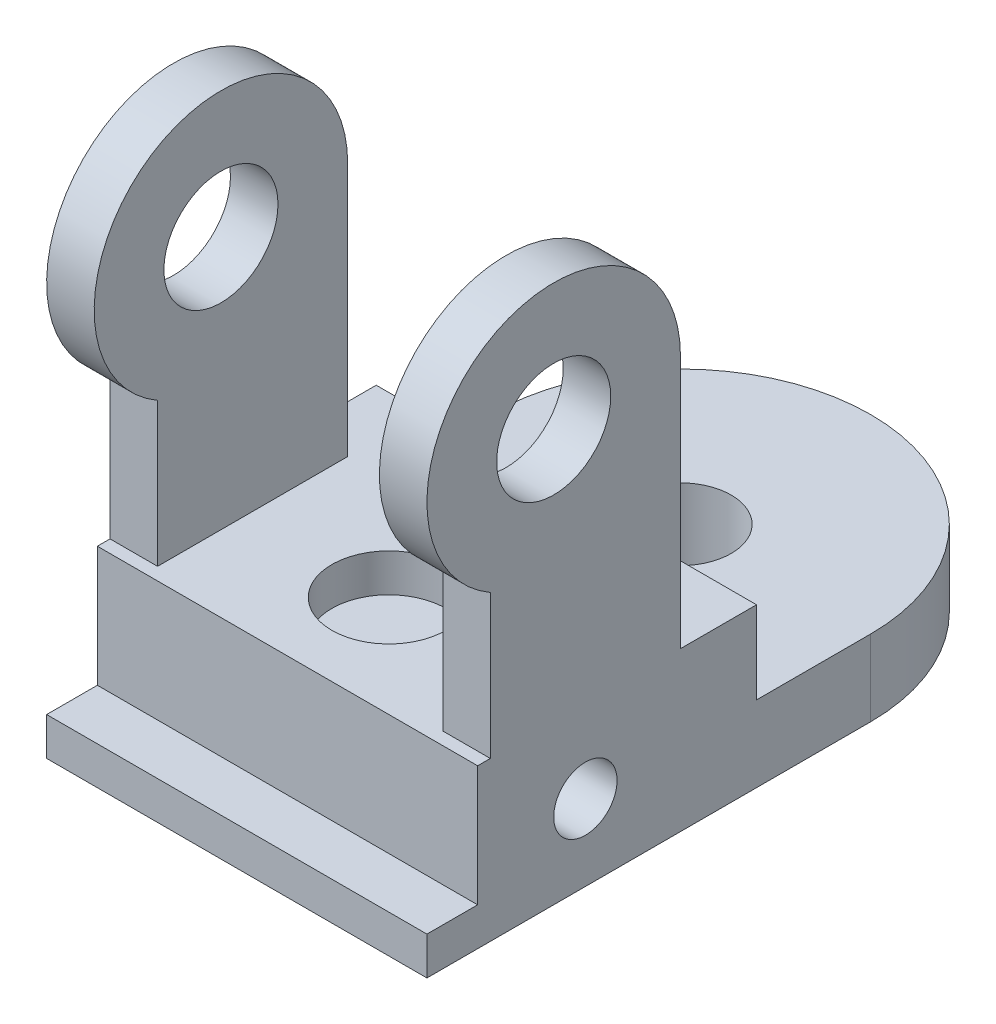
ISO-10303-21;
HEADER;
FILE_DESCRIPTION(('STEP AP214'),'2;1');
FILE_NAME('part.step','',(''),(''),'','','');
FILE_SCHEMA(('AUTOMOTIVE_DESIGN { 1 0 10303 214 1 1 1 1 }'));
ENDSEC;
DATA;
#1=APPLICATION_CONTEXT('core data for automotive mechanical design processes');
#2=APPLICATION_PROTOCOL_DEFINITION('international standard','automotive_design',2000,#1);
#3=PRODUCT_CONTEXT('',#1,'mechanical');
#4=PRODUCT('Part','Part','',(#3));
#5=PRODUCT_RELATED_PRODUCT_CATEGORY('part','',(#4));
#6=PRODUCT_DEFINITION_FORMATION('','',#4);
#7=PRODUCT_DEFINITION_CONTEXT('part definition',#1,'design');
#8=PRODUCT_DEFINITION('design','',#6,#7);
#9=PRODUCT_DEFINITION_SHAPE('','',#8);
#10=(LENGTH_UNIT() NAMED_UNIT(*) SI_UNIT(.MILLI.,.METRE.));
#11=(NAMED_UNIT(*) PLANE_ANGLE_UNIT() SI_UNIT($,.RADIAN.));
#12=(NAMED_UNIT(*) SI_UNIT($,.STERADIAN.) SOLID_ANGLE_UNIT());
#13=UNCERTAINTY_MEASURE_WITH_UNIT(LENGTH_MEASURE(1.E-05),#10,'distance_accuracy_value','');
#14=(GEOMETRIC_REPRESENTATION_CONTEXT(3) GLOBAL_UNCERTAINTY_ASSIGNED_CONTEXT((#13)) GLOBAL_UNIT_ASSIGNED_CONTEXT((#10,
#11,#12)) REPRESENTATION_CONTEXT('',''));
#15=CARTESIAN_POINT('',(0.,0.,0.));
#16=DIRECTION('',(0.,0.,1.));
#17=DIRECTION('',(1.,0.,0.));
#18=AXIS2_PLACEMENT_3D('',#15,#16,#17);
#19=CARTESIAN_POINT('',(-30.,0.,18.));
#20=DIRECTION('',(0.,0.,-1.));
#21=DIRECTION('',(-1.,0.,0.));
#22=AXIS2_PLACEMENT_3D('',#19,#20,#21);
#23=PLANE('',#22);
#24=CARTESIAN_POINT('',(0.,25.,18.));
#25=DIRECTION('',(0.,0.,-1.));
#26=DIRECTION('',(-1.,0.,0.));
#27=AXIS2_PLACEMENT_3D('',#24,#25,#26);
#28=CIRCLE('',#27,13.);
#29=CARTESIAN_POINT('',(13.,25.,18.));
#30=VERTEX_POINT('',#29);
#31=CARTESIAN_POINT('',(0.,12.,18.));
#32=VERTEX_POINT('',#31);
#33=EDGE_CURVE('E47',#30,#32,#28,.T.);
#34=ORIENTED_EDGE('',*,*,#33,.F.);
#35=DIRECTION('',(1.,0.,0.));
#36=VECTOR('',#35,1.);
#37=CARTESIAN_POINT('',(-30.,25.,18.));
#38=LINE('',#37,#36);
#39=CARTESIAN_POINT('',(30.,25.,18.));
#40=VERTEX_POINT('',#39);
#41=EDGE_CURVE('E183',#30,#40,#38,.T.);
#42=ORIENTED_EDGE('',*,*,#41,.T.);
#43=DIRECTION('',(0.,1.,0.));
#44=VECTOR('',#43,1.);
#45=CARTESIAN_POINT('',(30.,0.,18.));
#46=LINE('',#45,#44);
#47=CARTESIAN_POINT('',(30.,12.,18.));
#48=VERTEX_POINT('',#47);
#49=EDGE_CURVE('E252',#48,#40,#46,.T.);
#50=ORIENTED_EDGE('',*,*,#49,.F.);
#51=DIRECTION('',(1.,0.,0.));
#52=VECTOR('',#51,1.);
#53=CARTESIAN_POINT('',(-30.,12.,18.));
#54=LINE('',#53,#52);
#55=EDGE_CURVE('E261',#32,#48,#54,.T.);
#56=ORIENTED_EDGE('',*,*,#55,.F.);
#57=EDGE_LOOP('',(#34,#42,#50,#56));
#58=FACE_BOUND('',#57,.T.);
#59=ADVANCED_FACE('F41',(#58),#23,.T.);
#60=CARTESIAN_POINT('',(-30.,25.,0.));
#61=DIRECTION('',(0.,1.,0.));
#62=DIRECTION('',(0.,0.,1.));
#63=AXIS2_PLACEMENT_3D('',#60,#61,#62);
#64=PLANE('',#63);
#65=CARTESIAN_POINT('',(0.,25.,46.));
#66=DIRECTION('',(0.,1.,0.));
#67=DIRECTION('',(0.,0.,1.));
#68=AXIS2_PLACEMENT_3D('',#65,#66,#67);
#69=CIRCLE('',#68,9.);
#70=CARTESIAN_POINT('',(0.,25.,55.));
#71=VERTEX_POINT('',#70);
#72=EDGE_CURVE('E451',#71,#71,#69,.T.);
#73=ORIENTED_EDGE('',*,*,#72,.F.);
#74=EDGE_LOOP('',(#73));
#75=FACE_BOUND('',#74,.T.);
#76=DIRECTION('',(0.,0.,-1.));
#77=VECTOR('',#76,1.);
#78=CARTESIAN_POINT('',(13.,25.,30.));
#79=LINE('',#78,#77);
#80=CARTESIAN_POINT('',(13.,25.,30.));
#81=VERTEX_POINT('',#80);
#82=EDGE_CURVE('E174',#81,#30,#79,.T.);
#83=ORIENTED_EDGE('',*,*,#82,.F.);
#84=DIRECTION('',(-1.,0.,0.));
#85=VECTOR('',#84,1.);
#86=CARTESIAN_POINT('',(-30.,25.,30.));
#87=LINE('',#86,#85);
#88=CARTESIAN_POINT('',(-13.,25.,30.));
#89=VERTEX_POINT('',#88);
#90=EDGE_CURVE('E11',#81,#89,#87,.T.);
#91=ORIENTED_EDGE('',*,*,#90,.T.);
#92=DIRECTION('',(0.,0.,-1.));
#93=VECTOR('',#92,1.);
#94=CARTESIAN_POINT('',(-13.,25.,30.));
#95=LINE('',#94,#93);
#96=CARTESIAN_POINT('',(-13.,25.,18.));
#97=VERTEX_POINT('',#96);
#98=EDGE_CURVE('E166',#97,#89,#95,.F.);
#99=ORIENTED_EDGE('',*,*,#98,.F.);
#100=CARTESIAN_POINT('',(-30.,25.,18.));
#101=VERTEX_POINT('',#100);
#102=EDGE_CURVE('E273',#101,#97,#38,.T.);
#103=ORIENTED_EDGE('',*,*,#102,.F.);
#104=DIRECTION('',(0.,0.,1.));
#105=VECTOR('',#104,1.);
#106=CARTESIAN_POINT('',(-30.,25.,0.));
#107=LINE('',#106,#105);
#108=CARTESIAN_POINT('',(-30.,25.,30.));
#109=VERTEX_POINT('',#108);
#110=EDGE_CURVE('E262',#101,#109,#107,.T.);
#111=ORIENTED_EDGE('',*,*,#110,.T.);
#112=DIRECTION('',(-1.,0.,0.));
#113=VECTOR('',#112,1.);
#114=CARTESIAN_POINT('',(-22.5,25.,30.));
#115=LINE('',#114,#113);
#116=CARTESIAN_POINT('',(-22.5,25.,30.));
#117=VERTEX_POINT('',#116);
#118=EDGE_CURVE('E202',#117,#109,#115,.T.);
#119=ORIENTED_EDGE('',*,*,#118,.F.);
#120=DIRECTION('',(0.,0.,1.));
#121=VECTOR('',#120,1.);
#122=CARTESIAN_POINT('',(-22.5,25.,0.));
#123=LINE('',#122,#121);
#124=CARTESIAN_POINT('',(-22.5,25.,60.));
#125=VERTEX_POINT('',#124);
#126=EDGE_CURVE('E65',#117,#125,#123,.T.);
#127=ORIENTED_EDGE('',*,*,#126,.T.);
#128=DIRECTION('',(-1.,0.,0.));
#129=VECTOR('',#128,1.);
#130=CARTESIAN_POINT('',(-22.5,25.,60.));
#131=LINE('',#130,#129);
#132=CARTESIAN_POINT('',(-30.,25.,60.));
#133=VERTEX_POINT('',#132);
#134=EDGE_CURVE('E217',#125,#133,#131,.T.);
#135=ORIENTED_EDGE('',*,*,#134,.T.);
#136=CARTESIAN_POINT('',(-30.,25.,62.));
#137=VERTEX_POINT('',#136);
#138=EDGE_CURVE('E263',#133,#137,#107,.T.);
#139=ORIENTED_EDGE('',*,*,#138,.T.);
#140=DIRECTION('',(1.,0.,0.));
#141=VECTOR('',#140,1.);
#142=CARTESIAN_POINT('',(-30.,25.,62.));
#143=LINE('',#142,#141);
#144=CARTESIAN_POINT('',(30.,25.,62.));
#145=VERTEX_POINT('',#144);
#146=EDGE_CURVE('E272',#137,#145,#143,.T.);
#147=ORIENTED_EDGE('',*,*,#146,.T.);
#148=DIRECTION('',(0.,0.,1.));
#149=VECTOR('',#148,1.);
#150=CARTESIAN_POINT('',(30.,25.,0.));
#151=LINE('',#150,#149);
#152=CARTESIAN_POINT('',(30.,25.,60.));
#153=VERTEX_POINT('',#152);
#154=EDGE_CURVE('E267',#153,#145,#151,.T.);
#155=ORIENTED_EDGE('',*,*,#154,.F.);
#156=DIRECTION('',(1.,0.,0.));
#157=VECTOR('',#156,1.);
#158=CARTESIAN_POINT('',(22.5,25.,60.));
#159=LINE('',#158,#157);
#160=CARTESIAN_POINT('',(22.5,25.,60.));
#161=VERTEX_POINT('',#160);
#162=EDGE_CURVE('E255',#161,#153,#159,.T.);
#163=ORIENTED_EDGE('',*,*,#162,.F.);
#164=DIRECTION('',(0.,0.,1.));
#165=VECTOR('',#164,1.);
#166=CARTESIAN_POINT('',(22.5,25.,0.));
#167=LINE('',#166,#165);
#168=CARTESIAN_POINT('',(22.5,25.,30.));
#169=VERTEX_POINT('',#168);
#170=EDGE_CURVE('E234',#169,#161,#167,.T.);
#171=ORIENTED_EDGE('',*,*,#170,.F.);
#172=DIRECTION('',(1.,0.,0.));
#173=VECTOR('',#172,1.);
#174=CARTESIAN_POINT('',(22.5,25.,30.));
#175=LINE('',#174,#173);
#176=CARTESIAN_POINT('',(30.,25.,30.));
#177=VERTEX_POINT('',#176);
#178=EDGE_CURVE('E247',#169,#177,#175,.T.);
#179=ORIENTED_EDGE('',*,*,#178,.T.);
#180=EDGE_CURVE('E264',#40,#177,#151,.T.);
#181=ORIENTED_EDGE('',*,*,#180,.F.);
#182=ORIENTED_EDGE('',*,*,#41,.F.);
#183=EDGE_LOOP('',(#83,#91,#99,#103,#111,#119,#127,#135,#139,#147,#155,#163,#171,#179,#181,#182));
#184=FACE_BOUND('',#183,.T.);
#185=ADVANCED_FACE('F181',(#75,#184),#64,.T.);
#186=CARTESIAN_POINT('',(0.,12.,0.));
#187=DIRECTION('',(0.,1.,0.));
#188=DIRECTION('',(0.,0.,1.));
#189=AXIS2_PLACEMENT_3D('',#186,#187,#188);
#190=PLANE('',#189);
#191=CARTESIAN_POINT('',(0.,12.,0.));
#192=DIRECTION('',(0.,1.,0.));
#193=DIRECTION('',(0.,0.,1.));
#194=AXIS2_PLACEMENT_3D('',#191,#192,#193);
#195=CIRCLE('',#194,8.);
#196=CARTESIAN_POINT('',(0.,12.,8.));
#197=VERTEX_POINT('',#196);
#198=EDGE_CURVE('E292',#197,#197,#195,.T.);
#199=ORIENTED_EDGE('',*,*,#198,.F.);
#200=EDGE_LOOP('',(#199));
#201=FACE_BOUND('',#200,.T.);
#202=DIRECTION('',(0.,0.,1.));
#203=VECTOR('',#202,1.);
#204=CARTESIAN_POINT('',(-30.,12.,70.));
#205=LINE('',#204,#203);
#206=CARTESIAN_POINT('',(-30.,12.,0.));
#207=VERTEX_POINT('',#206);
#208=CARTESIAN_POINT('',(-30.,12.,18.));
#209=VERTEX_POINT('',#208);
#210=EDGE_CURVE('E302',#207,#209,#205,.T.);
#211=ORIENTED_EDGE('',*,*,#210,.T.);
#212=EDGE_CURVE('E276',#209,#32,#54,.T.);
#213=ORIENTED_EDGE('',*,*,#212,.T.);
#214=ORIENTED_EDGE('',*,*,#55,.T.);
#215=DIRECTION('',(0.,0.,-1.));
#216=VECTOR('',#215,1.);
#217=CARTESIAN_POINT('',(30.,12.,0.));
#218=LINE('',#217,#216);
#219=CARTESIAN_POINT('',(30.,12.,0.));
#220=VERTEX_POINT('',#219);
#221=EDGE_CURVE('E308',#48,#220,#218,.T.);
#222=ORIENTED_EDGE('',*,*,#221,.T.);
#223=CARTESIAN_POINT('',(0.,12.,0.));
#224=DIRECTION('',(0.,1.,0.));
#225=DIRECTION('',(0.,0.,1.));
#226=AXIS2_PLACEMENT_3D('',#223,#224,#225);
#227=CIRCLE('',#226,30.);
#228=EDGE_CURVE('E301',#220,#207,#227,.T.);
#229=ORIENTED_EDGE('',*,*,#228,.T.);
#230=EDGE_LOOP('',(#211,#213,#214,#222,#229));
#231=FACE_BOUND('',#230,.T.);
#232=ADVANCED_FACE('F378',(#201,#231),#190,.T.);
#233=CARTESIAN_POINT('',(30.,12.,70.));
#234=DIRECTION('',(0.,0.,-1.));
#235=DIRECTION('',(-1.,0.,0.));
#236=AXIS2_PLACEMENT_3D('',#233,#234,#235);
#237=PLANE('',#236);
#238=DIRECTION('',(1.,0.,0.));
#239=VECTOR('',#238,1.);
#240=CARTESIAN_POINT('',(-30.,6.,70.));
#241=LINE('',#240,#239);
#242=CARTESIAN_POINT('',(-30.,6.,70.));
#243=VERTEX_POINT('',#242);
#244=CARTESIAN_POINT('',(30.,6.,70.));
#245=VERTEX_POINT('',#244);
#246=EDGE_CURVE('E283',#243,#245,#241,.T.);
#247=ORIENTED_EDGE('',*,*,#246,.F.);
#248=DIRECTION('',(0.,-1.,0.));
#249=VECTOR('',#248,1.);
#250=CARTESIAN_POINT('',(-30.,12.,70.));
#251=LINE('',#250,#249);
#252=CARTESIAN_POINT('',(-30.,0.,70.));
#253=VERTEX_POINT('',#252);
#254=EDGE_CURVE('E323',#243,#253,#251,.T.);
#255=ORIENTED_EDGE('',*,*,#254,.T.);
#256=DIRECTION('',(1.,0.,0.));
#257=VECTOR('',#256,1.);
#258=CARTESIAN_POINT('',(30.,0.,70.));
#259=LINE('',#258,#257);
#260=CARTESIAN_POINT('',(30.,0.,70.));
#261=VERTEX_POINT('',#260);
#262=EDGE_CURVE('E317',#253,#261,#259,.T.);
#263=ORIENTED_EDGE('',*,*,#262,.T.);
#264=DIRECTION('',(0.,-1.,0.));
#265=VECTOR('',#264,1.);
#266=CARTESIAN_POINT('',(30.,12.,70.));
#267=LINE('',#266,#265);
#268=EDGE_CURVE('E321',#245,#261,#267,.T.);
#269=ORIENTED_EDGE('',*,*,#268,.F.);
#270=EDGE_LOOP('',(#247,#255,#263,#269));
#271=FACE_BOUND('',#270,.T.);
#272=ADVANCED_FACE('F348',(#271),#237,.F.);
#273=CARTESIAN_POINT('',(0.,12.,0.));
#274=DIRECTION('',(0.,-1.,0.));
#275=DIRECTION('',(0.,0.,-1.));
#276=AXIS2_PLACEMENT_3D('',#273,#274,#275);
#277=CYLINDRICAL_SURFACE('',#276,30.);
#278=CARTESIAN_POINT('',(0.,0.,0.));
#279=DIRECTION('',(0.,1.,0.));
#280=DIRECTION('',(0.,0.,1.));
#281=AXIS2_PLACEMENT_3D('',#278,#279,#280);
#282=CIRCLE('',#281,30.);
#283=CARTESIAN_POINT('',(30.,0.,0.));
#284=VERTEX_POINT('',#283);
#285=CARTESIAN_POINT('',(-30.,0.,0.));
#286=VERTEX_POINT('',#285);
#287=EDGE_CURVE('E296',#284,#286,#282,.T.);
#288=ORIENTED_EDGE('',*,*,#287,.T.);
#289=DIRECTION('',(0.,-1.,0.));
#290=VECTOR('',#289,1.);
#291=CARTESIAN_POINT('',(-30.,12.,0.));
#292=LINE('',#291,#290);
#293=EDGE_CURVE('E328',#207,#286,#292,.T.);
#294=ORIENTED_EDGE('',*,*,#293,.F.);
#295=ORIENTED_EDGE('',*,*,#228,.F.);
#296=DIRECTION('',(0.,-1.,0.));
#297=VECTOR('',#296,1.);
#298=CARTESIAN_POINT('',(30.,12.,0.));
#299=LINE('',#298,#297);
#300=EDGE_CURVE('E309',#220,#284,#299,.T.);
#301=ORIENTED_EDGE('',*,*,#300,.T.);
#302=EDGE_LOOP('',(#288,#294,#295,#301));
#303=FACE_BOUND('',#302,.T.);
#304=ADVANCED_FACE('F43',(#303),#277,.T.);
#305=CARTESIAN_POINT('',(-30.,12.,70.));
#306=DIRECTION('',(1.,0.,0.));
#307=DIRECTION('',(0.,0.,-1.));
#308=AXIS2_PLACEMENT_3D('',#305,#306,#307);
#309=PLANE('',#308);
#310=CARTESIAN_POINT('',(-30.,12.,45.));
#311=DIRECTION('',(-1.,0.,0.));
#312=DIRECTION('',(0.,0.,1.));
#313=AXIS2_PLACEMENT_3D('',#310,#311,#312);
#314=CIRCLE('',#313,5.);
#315=CARTESIAN_POINT('',(-30.,12.,50.));
#316=VERTEX_POINT('',#315);
#317=EDGE_CURVE('E450',#316,#316,#314,.T.);
#318=ORIENTED_EDGE('',*,*,#317,.F.);
#319=EDGE_LOOP('',(#318));
#320=FACE_BOUND('',#319,.T.);
#321=DIRECTION('',(0.,0.,1.));
#322=VECTOR('',#321,1.);
#323=CARTESIAN_POINT('',(-30.,6.,62.));
#324=LINE('',#323,#322);
#325=CARTESIAN_POINT('',(-30.,6.,62.));
#326=VERTEX_POINT('',#325);
#327=EDGE_CURVE('E274',#326,#243,#324,.T.);
#328=ORIENTED_EDGE('',*,*,#327,.F.);
#329=DIRECTION('',(0.,1.,0.));
#330=VECTOR('',#329,1.);
#331=CARTESIAN_POINT('',(-30.,6.,62.));
#332=LINE('',#331,#330);
#333=EDGE_CURVE('E290',#326,#137,#332,.T.);
#334=ORIENTED_EDGE('',*,*,#333,.T.);
#335=ORIENTED_EDGE('',*,*,#138,.F.);
#336=DIRECTION('',(0.,1.,0.));
#337=VECTOR('',#336,1.);
#338=CARTESIAN_POINT('',(-30.,0.,60.));
#339=LINE('',#338,#337);
#340=CARTESIAN_POINT('',(-30.,47.6794919243112,60.));
#341=VERTEX_POINT('',#340);
#342=EDGE_CURVE('E210',#133,#341,#339,.T.);
#343=ORIENTED_EDGE('',*,*,#342,.T.);
#344=CARTESIAN_POINT('',(-30.,65.,50.));
#345=DIRECTION('',(1.,0.,0.));
#346=DIRECTION('',(0.,0.,-1.));
#347=AXIS2_PLACEMENT_3D('',#344,#345,#346);
#348=CIRCLE('',#347,20.);
#349=CARTESIAN_POINT('',(-30.,65.,30.));
#350=VERTEX_POINT('',#349);
#351=EDGE_CURVE('E192',#350,#341,#348,.T.);
#352=ORIENTED_EDGE('',*,*,#351,.F.);
#353=DIRECTION('',(0.,1.,0.));
#354=VECTOR('',#353,1.);
#355=CARTESIAN_POINT('',(-30.,0.,30.));
#356=LINE('',#355,#354);
#357=EDGE_CURVE('E189',#109,#350,#356,.T.);
#358=ORIENTED_EDGE('',*,*,#357,.F.);
#359=ORIENTED_EDGE('',*,*,#110,.F.);
#360=DIRECTION('',(0.,1.,0.));
#361=VECTOR('',#360,1.);
#362=CARTESIAN_POINT('',(-30.,0.,18.));
#363=LINE('',#362,#361);
#364=EDGE_CURVE('E260',#209,#101,#363,.T.);
#365=ORIENTED_EDGE('',*,*,#364,.F.);
#366=ORIENTED_EDGE('',*,*,#210,.F.);
#367=ORIENTED_EDGE('',*,*,#293,.T.);
#368=DIRECTION('',(0.,0.,1.));
#369=VECTOR('',#368,1.);
#370=CARTESIAN_POINT('',(-30.,0.,70.));
#371=LINE('',#370,#369);
#372=EDGE_CURVE('E312',#286,#253,#371,.T.);
#373=ORIENTED_EDGE('',*,*,#372,.T.);
#374=ORIENTED_EDGE('',*,*,#254,.F.);
#375=EDGE_LOOP('',(#328,#334,#335,#343,#352,#358,#359,#365,#366,#367,#373,#374));
#376=FACE_BOUND('',#375,.T.);
#377=CARTESIAN_POINT('',(-30.,65.,50.));
#378=DIRECTION('',(1.,0.,0.));
#379=DIRECTION('',(0.,0.,-1.));
#380=AXIS2_PLACEMENT_3D('',#377,#378,#379);
#381=CIRCLE('',#380,9.00000000000001);
#382=CARTESIAN_POINT('',(-30.,65.,41.));
#383=VERTEX_POINT('',#382);
#384=EDGE_CURVE('E184',#383,#383,#381,.T.);
#385=ORIENTED_EDGE('',*,*,#384,.T.);
#386=EDGE_LOOP('',(#385));
#387=FACE_BOUND('',#386,.T.);
#388=ADVANCED_FACE('F333',(#320,#376,#387),#309,.F.);
#389=CARTESIAN_POINT('',(30.,12.,0.));
#390=DIRECTION('',(-1.,0.,0.));
#391=DIRECTION('',(0.,0.,1.));
#392=AXIS2_PLACEMENT_3D('',#389,#390,#391);
#393=PLANE('',#392);
#394=CARTESIAN_POINT('',(30.,12.,45.));
#395=DIRECTION('',(1.,0.,0.));
#396=DIRECTION('',(0.,0.,-1.));
#397=AXIS2_PLACEMENT_3D('',#394,#395,#396);
#398=CIRCLE('',#397,5.);
#399=CARTESIAN_POINT('',(30.,12.,40.));
#400=VERTEX_POINT('',#399);
#401=EDGE_CURVE('E446',#400,#400,#398,.T.);
#402=ORIENTED_EDGE('',*,*,#401,.F.);
#403=EDGE_LOOP('',(#402));
#404=FACE_BOUND('',#403,.T.);
#405=ORIENTED_EDGE('',*,*,#221,.F.);
#406=ORIENTED_EDGE('',*,*,#49,.T.);
#407=ORIENTED_EDGE('',*,*,#180,.T.);
#408=DIRECTION('',(0.,1.,0.));
#409=VECTOR('',#408,1.);
#410=CARTESIAN_POINT('',(30.,0.,30.));
#411=LINE('',#410,#409);
#412=CARTESIAN_POINT('',(30.,65.,30.));
#413=VERTEX_POINT('',#412);
#414=EDGE_CURVE('E239',#177,#413,#411,.T.);
#415=ORIENTED_EDGE('',*,*,#414,.T.);
#416=CARTESIAN_POINT('',(30.,65.,50.));
#417=DIRECTION('',(1.,0.,0.));
#418=DIRECTION('',(0.,0.,-1.));
#419=AXIS2_PLACEMENT_3D('',#416,#417,#418);
#420=CIRCLE('',#419,20.);
#421=CARTESIAN_POINT('',(30.,47.6794919243112,60.));
#422=VERTEX_POINT('',#421);
#423=EDGE_CURVE('E243',#413,#422,#420,.T.);
#424=ORIENTED_EDGE('',*,*,#423,.T.);
#425=DIRECTION('',(0.,1.,0.));
#426=VECTOR('',#425,1.);
#427=CARTESIAN_POINT('',(30.,0.,60.));
#428=LINE('',#427,#426);
#429=EDGE_CURVE('E228',#153,#422,#428,.T.);
#430=ORIENTED_EDGE('',*,*,#429,.F.);
#431=ORIENTED_EDGE('',*,*,#154,.T.);
#432=DIRECTION('',(0.,1.,0.));
#433=VECTOR('',#432,1.);
#434=CARTESIAN_POINT('',(30.,6.,62.));
#435=LINE('',#434,#433);
#436=CARTESIAN_POINT('',(30.,6.,62.));
#437=VERTEX_POINT('',#436);
#438=EDGE_CURVE('E287',#437,#145,#435,.T.);
#439=ORIENTED_EDGE('',*,*,#438,.F.);
#440=DIRECTION('',(0.,0.,-1.));
#441=VECTOR('',#440,1.);
#442=CARTESIAN_POINT('',(30.,6.,70.));
#443=LINE('',#442,#441);
#444=EDGE_CURVE('E282',#245,#437,#443,.T.);
#445=ORIENTED_EDGE('',*,*,#444,.F.);
#446=ORIENTED_EDGE('',*,*,#268,.T.);
#447=DIRECTION('',(0.,0.,-1.));
#448=VECTOR('',#447,1.);
#449=CARTESIAN_POINT('',(30.,0.,0.));
#450=LINE('',#449,#448);
#451=EDGE_CURVE('E304',#261,#284,#450,.T.);
#452=ORIENTED_EDGE('',*,*,#451,.T.);
#453=ORIENTED_EDGE('',*,*,#300,.F.);
#454=EDGE_LOOP('',(#405,#406,#407,#415,#424,#430,#431,#439,#445,#446,#452,#453));
#455=FACE_BOUND('',#454,.T.);
#456=CARTESIAN_POINT('',(30.,65.,50.));
#457=DIRECTION('',(1.,0.,0.));
#458=DIRECTION('',(0.,0.,-1.));
#459=AXIS2_PLACEMENT_3D('',#456,#457,#458);
#460=CIRCLE('',#459,9.00000000000001);
#461=CARTESIAN_POINT('',(30.,65.,41.));
#462=VERTEX_POINT('',#461);
#463=EDGE_CURVE('E212',#462,#462,#460,.T.);
#464=ORIENTED_EDGE('',*,*,#463,.F.);
#465=EDGE_LOOP('',(#464));
#466=FACE_BOUND('',#465,.T.);
#467=ADVANCED_FACE('F357',(#404,#455,#466),#393,.F.);
#468=CARTESIAN_POINT('',(0.,0.,0.));
#469=DIRECTION('',(0.,1.,0.));
#470=DIRECTION('',(0.,0.,1.));
#471=AXIS2_PLACEMENT_3D('',#468,#469,#470);
#472=PLANE('',#471);
#473=CARTESIAN_POINT('',(0.,0.,0.));
#474=DIRECTION('',(0.,1.,0.));
#475=DIRECTION('',(0.,0.,1.));
#476=AXIS2_PLACEMENT_3D('',#473,#474,#475);
#477=CIRCLE('',#476,8.);
#478=CARTESIAN_POINT('',(0.,0.,8.));
#479=VERTEX_POINT('',#478);
#480=EDGE_CURVE('E294',#479,#479,#477,.T.);
#481=ORIENTED_EDGE('',*,*,#480,.T.);
#482=EDGE_LOOP('',(#481));
#483=FACE_BOUND('',#482,.T.);
#484=ORIENTED_EDGE('',*,*,#287,.F.);
#485=ORIENTED_EDGE('',*,*,#451,.F.);
#486=ORIENTED_EDGE('',*,*,#262,.F.);
#487=ORIENTED_EDGE('',*,*,#372,.F.);
#488=EDGE_LOOP('',(#484,#485,#486,#487));
#489=FACE_BOUND('',#488,.T.);
#490=ADVANCED_FACE('F341',(#483,#489),#472,.F.);
#491=CARTESIAN_POINT('',(0.,0.,0.));
#492=DIRECTION('',(0.,1.,0.));
#493=DIRECTION('',(0.,0.,1.));
#494=AXIS2_PLACEMENT_3D('',#491,#492,#493);
#495=CYLINDRICAL_SURFACE('',#494,8.);
#496=ORIENTED_EDGE('',*,*,#480,.F.);
#497=EDGE_LOOP('',(#496));
#498=FACE_BOUND('',#497,.T.);
#499=ORIENTED_EDGE('',*,*,#198,.T.);
#500=EDGE_LOOP('',(#499));
#501=FACE_BOUND('',#500,.T.);
#502=ADVANCED_FACE('F424',(#498,#501),#495,.F.);
#503=CARTESIAN_POINT('',(30.,6.,62.));
#504=DIRECTION('',(0.,0.,-1.));
#505=DIRECTION('',(-1.,0.,0.));
#506=AXIS2_PLACEMENT_3D('',#503,#504,#505);
#507=PLANE('',#506);
#508=ORIENTED_EDGE('',*,*,#438,.T.);
#509=ORIENTED_EDGE('',*,*,#146,.F.);
#510=ORIENTED_EDGE('',*,*,#333,.F.);
#511=DIRECTION('',(-1.,0.,0.));
#512=VECTOR('',#511,1.);
#513=CARTESIAN_POINT('',(30.,6.,62.));
#514=LINE('',#513,#512);
#515=EDGE_CURVE('E281',#437,#326,#514,.T.);
#516=ORIENTED_EDGE('',*,*,#515,.F.);
#517=EDGE_LOOP('',(#508,#509,#510,#516));
#518=FACE_BOUND('',#517,.T.);
#519=ADVANCED_FACE('F355',(#518),#507,.F.);
#520=CARTESIAN_POINT('',(0.,6.,0.));
#521=DIRECTION('',(0.,1.,0.));
#522=DIRECTION('',(0.,0.,1.));
#523=AXIS2_PLACEMENT_3D('',#520,#521,#522);
#524=PLANE('',#523);
#525=ORIENTED_EDGE('',*,*,#327,.T.);
#526=ORIENTED_EDGE('',*,*,#246,.T.);
#527=ORIENTED_EDGE('',*,*,#444,.T.);
#528=ORIENTED_EDGE('',*,*,#515,.T.);
#529=EDGE_LOOP('',(#525,#526,#527,#528));
#530=FACE_BOUND('',#529,.T.);
#531=ADVANCED_FACE('F350',(#530),#524,.T.);
#532=EDGE_CURVE('E173',#32,#97,#28,.T.);
#533=ORIENTED_EDGE('',*,*,#532,.F.);
#534=ORIENTED_EDGE('',*,*,#212,.F.);
#535=ORIENTED_EDGE('',*,*,#364,.T.);
#536=ORIENTED_EDGE('',*,*,#102,.T.);
#537=EDGE_LOOP('',(#533,#534,#535,#536));
#538=FACE_BOUND('',#537,.T.);
#539=ADVANCED_FACE('F376',(#538),#23,.T.);
#540=CARTESIAN_POINT('',(22.5,0.,30.));
#541=DIRECTION('',(0.,0.,-1.));
#542=DIRECTION('',(-1.,0.,0.));
#543=AXIS2_PLACEMENT_3D('',#540,#541,#542);
#544=PLANE('',#543);
#545=ORIENTED_EDGE('',*,*,#414,.F.);
#546=ORIENTED_EDGE('',*,*,#178,.F.);
#547=DIRECTION('',(0.,1.,0.));
#548=VECTOR('',#547,1.);
#549=CARTESIAN_POINT('',(22.5,0.,30.));
#550=LINE('',#549,#548);
#551=CARTESIAN_POINT('',(22.5,65.,30.));
#552=VERTEX_POINT('',#551);
#553=EDGE_CURVE('E221',#169,#552,#550,.T.);
#554=ORIENTED_EDGE('',*,*,#553,.T.);
#555=DIRECTION('',(1.,0.,0.));
#556=VECTOR('',#555,1.);
#557=CARTESIAN_POINT('',(22.5,65.,30.));
#558=LINE('',#557,#556);
#559=EDGE_CURVE('E240',#552,#413,#558,.T.);
#560=ORIENTED_EDGE('',*,*,#559,.T.);
#561=EDGE_LOOP('',(#545,#546,#554,#560));
#562=FACE_BOUND('',#561,.T.);
#563=ADVANCED_FACE('F381',(#562),#544,.T.);
#564=CARTESIAN_POINT('',(22.5,0.,60.));
#565=DIRECTION('',(0.,0.,-1.));
#566=DIRECTION('',(-1.,0.,0.));
#567=AXIS2_PLACEMENT_3D('',#564,#565,#566);
#568=PLANE('',#567);
#569=ORIENTED_EDGE('',*,*,#429,.T.);
#570=DIRECTION('',(1.,0.,0.));
#571=VECTOR('',#570,1.);
#572=CARTESIAN_POINT('',(22.5,47.6794919243112,60.));
#573=LINE('',#572,#571);
#574=CARTESIAN_POINT('',(22.5,47.6794919243112,60.));
#575=VERTEX_POINT('',#574);
#576=EDGE_CURVE('E253',#575,#422,#573,.T.);
#577=ORIENTED_EDGE('',*,*,#576,.F.);
#578=DIRECTION('',(0.,1.,0.));
#579=VECTOR('',#578,1.);
#580=CARTESIAN_POINT('',(22.5,0.,60.));
#581=LINE('',#580,#579);
#582=EDGE_CURVE('E235',#161,#575,#581,.T.);
#583=ORIENTED_EDGE('',*,*,#582,.F.);
#584=ORIENTED_EDGE('',*,*,#162,.T.);
#585=EDGE_LOOP('',(#569,#577,#583,#584));
#586=FACE_BOUND('',#585,.T.);
#587=ADVANCED_FACE('F392',(#586),#568,.F.);
#588=CARTESIAN_POINT('',(22.5,65.,50.));
#589=DIRECTION('',(1.,0.,0.));
#590=DIRECTION('',(0.,0.,-1.));
#591=AXIS2_PLACEMENT_3D('',#588,#589,#590);
#592=CYLINDRICAL_SURFACE('',#591,9.00000000000001);
#593=CARTESIAN_POINT('',(22.5,65.,50.));
#594=DIRECTION('',(1.,0.,0.));
#595=DIRECTION('',(0.,0.,-1.));
#596=AXIS2_PLACEMENT_3D('',#593,#594,#595);
#597=CIRCLE('',#596,9.00000000000001);
#598=CARTESIAN_POINT('',(22.5,65.,41.));
#599=VERTEX_POINT('',#598);
#600=EDGE_CURVE('E224',#599,#599,#597,.T.);
#601=ORIENTED_EDGE('',*,*,#600,.F.);
#602=EDGE_LOOP('',(#601));
#603=FACE_BOUND('',#602,.T.);
#604=ORIENTED_EDGE('',*,*,#463,.T.);
#605=EDGE_LOOP('',(#604));
#606=FACE_BOUND('',#605,.T.);
#607=ADVANCED_FACE('F391',(#603,#606),#592,.F.);
#608=CARTESIAN_POINT('',(22.5,65.,50.));
#609=DIRECTION('',(1.,0.,0.));
#610=DIRECTION('',(0.,0.,-1.));
#611=AXIS2_PLACEMENT_3D('',#608,#609,#610);
#612=CYLINDRICAL_SURFACE('',#611,20.);
#613=ORIENTED_EDGE('',*,*,#423,.F.);
#614=ORIENTED_EDGE('',*,*,#559,.F.);
#615=CARTESIAN_POINT('',(22.5,65.,50.));
#616=DIRECTION('',(1.,0.,0.));
#617=DIRECTION('',(0.,0.,-1.));
#618=AXIS2_PLACEMENT_3D('',#615,#616,#617);
#619=CIRCLE('',#618,20.);
#620=EDGE_CURVE('E230',#552,#575,#619,.T.);
#621=ORIENTED_EDGE('',*,*,#620,.T.);
#622=ORIENTED_EDGE('',*,*,#576,.T.);
#623=EDGE_LOOP('',(#613,#614,#621,#622));
#624=FACE_BOUND('',#623,.T.);
#625=ADVANCED_FACE('F393',(#624),#612,.T.);
#626=CARTESIAN_POINT('',(22.5,0.,0.));
#627=DIRECTION('',(1.,0.,0.));
#628=DIRECTION('',(0.,0.,-1.));
#629=AXIS2_PLACEMENT_3D('',#626,#627,#628);
#630=PLANE('',#629);
#631=ORIENTED_EDGE('',*,*,#600,.T.);
#632=EDGE_LOOP('',(#631));
#633=FACE_BOUND('',#632,.T.);
#634=ORIENTED_EDGE('',*,*,#553,.F.);
#635=ORIENTED_EDGE('',*,*,#170,.T.);
#636=ORIENTED_EDGE('',*,*,#582,.T.);
#637=ORIENTED_EDGE('',*,*,#620,.F.);
#638=EDGE_LOOP('',(#634,#635,#636,#637));
#639=FACE_BOUND('',#638,.T.);
#640=ADVANCED_FACE('F386',(#633,#639),#630,.F.);
#641=CARTESIAN_POINT('',(-22.5,0.,30.));
#642=DIRECTION('',(0.,0.,1.));
#643=DIRECTION('',(1.,0.,0.));
#644=AXIS2_PLACEMENT_3D('',#641,#642,#643);
#645=PLANE('',#644);
#646=ORIENTED_EDGE('',*,*,#357,.T.);
#647=DIRECTION('',(-1.,0.,0.));
#648=VECTOR('',#647,1.);
#649=CARTESIAN_POINT('',(-22.5,65.,30.));
#650=LINE('',#649,#648);
#651=CARTESIAN_POINT('',(-22.5,65.,30.));
#652=VERTEX_POINT('',#651);
#653=EDGE_CURVE('E211',#652,#350,#650,.T.);
#654=ORIENTED_EDGE('',*,*,#653,.F.);
#655=DIRECTION('',(0.,1.,0.));
#656=VECTOR('',#655,1.);
#657=CARTESIAN_POINT('',(-22.5,0.,30.));
#658=LINE('',#657,#656);
#659=EDGE_CURVE('E193',#117,#652,#658,.T.);
#660=ORIENTED_EDGE('',*,*,#659,.F.);
#661=ORIENTED_EDGE('',*,*,#118,.T.);
#662=EDGE_LOOP('',(#646,#654,#660,#661));
#663=FACE_BOUND('',#662,.T.);
#664=ADVANCED_FACE('F373',(#663),#645,.F.);
#665=CARTESIAN_POINT('',(-22.5,65.,50.));
#666=DIRECTION('',(-1.,0.,0.));
#667=DIRECTION('',(0.,0.,1.));
#668=AXIS2_PLACEMENT_3D('',#665,#666,#667);
#669=CYLINDRICAL_SURFACE('',#668,20.);
#670=ORIENTED_EDGE('',*,*,#351,.T.);
#671=DIRECTION('',(-1.,0.,0.));
#672=VECTOR('',#671,1.);
#673=CARTESIAN_POINT('',(-22.5,47.6794919243112,60.));
#674=LINE('',#673,#672);
#675=CARTESIAN_POINT('',(-22.5,47.6794919243112,60.));
#676=VERTEX_POINT('',#675);
#677=EDGE_CURVE('E218',#676,#341,#674,.T.);
#678=ORIENTED_EDGE('',*,*,#677,.F.);
#679=CARTESIAN_POINT('',(-22.5,65.,50.));
#680=DIRECTION('',(1.,0.,0.));
#681=DIRECTION('',(0.,0.,-1.));
#682=AXIS2_PLACEMENT_3D('',#679,#680,#681);
#683=CIRCLE('',#682,20.);
#684=EDGE_CURVE('E204',#652,#676,#683,.T.);
#685=ORIENTED_EDGE('',*,*,#684,.F.);
#686=ORIENTED_EDGE('',*,*,#653,.T.);
#687=EDGE_LOOP('',(#670,#678,#685,#686));
#688=FACE_BOUND('',#687,.T.);
#689=ADVANCED_FACE('F367',(#688),#669,.T.);
#690=CARTESIAN_POINT('',(-22.5,0.,60.));
#691=DIRECTION('',(0.,0.,1.));
#692=DIRECTION('',(1.,0.,0.));
#693=AXIS2_PLACEMENT_3D('',#690,#691,#692);
#694=PLANE('',#693);
#695=ORIENTED_EDGE('',*,*,#342,.F.);
#696=ORIENTED_EDGE('',*,*,#134,.F.);
#697=DIRECTION('',(0.,1.,0.));
#698=VECTOR('',#697,1.);
#699=CARTESIAN_POINT('',(-22.5,0.,60.));
#700=LINE('',#699,#698);
#701=EDGE_CURVE('E200',#125,#676,#700,.T.);
#702=ORIENTED_EDGE('',*,*,#701,.T.);
#703=ORIENTED_EDGE('',*,*,#677,.T.);
#704=EDGE_LOOP('',(#695,#696,#702,#703));
#705=FACE_BOUND('',#704,.T.);
#706=ADVANCED_FACE('F362',(#705),#694,.T.);
#707=CARTESIAN_POINT('',(-22.5,65.,50.));
#708=DIRECTION('',(-1.,0.,0.));
#709=DIRECTION('',(0.,0.,1.));
#710=AXIS2_PLACEMENT_3D('',#707,#708,#709);
#711=CYLINDRICAL_SURFACE('',#710,9.00000000000001);
#712=CARTESIAN_POINT('',(-22.5,65.,50.));
#713=DIRECTION('',(1.,0.,0.));
#714=DIRECTION('',(0.,0.,-1.));
#715=AXIS2_PLACEMENT_3D('',#712,#713,#714);
#716=CIRCLE('',#715,9.00000000000001);
#717=CARTESIAN_POINT('',(-22.5,65.,41.));
#718=VERTEX_POINT('',#717);
#719=EDGE_CURVE('E194',#718,#718,#716,.T.);
#720=ORIENTED_EDGE('',*,*,#719,.T.);
#721=EDGE_LOOP('',(#720));
#722=FACE_BOUND('',#721,.T.);
#723=ORIENTED_EDGE('',*,*,#384,.F.);
#724=EDGE_LOOP('',(#723));
#725=FACE_BOUND('',#724,.T.);
#726=ADVANCED_FACE('F480',(#722,#725),#711,.F.);
#727=CARTESIAN_POINT('',(-22.5,0.,0.));
#728=DIRECTION('',(-1.,0.,0.));
#729=DIRECTION('',(0.,0.,-1.));
#730=AXIS2_PLACEMENT_3D('',#727,#728,#729);
#731=PLANE('',#730);
#732=ORIENTED_EDGE('',*,*,#719,.F.);
#733=EDGE_LOOP('',(#732));
#734=FACE_BOUND('',#733,.T.);
#735=ORIENTED_EDGE('',*,*,#659,.T.);
#736=ORIENTED_EDGE('',*,*,#684,.T.);
#737=ORIENTED_EDGE('',*,*,#701,.F.);
#738=ORIENTED_EDGE('',*,*,#126,.F.);
#739=EDGE_LOOP('',(#735,#736,#737,#738));
#740=FACE_BOUND('',#739,.T.);
#741=ADVANCED_FACE('F479',(#734,#740),#731,.F.);
#742=CARTESIAN_POINT('',(0.,25.,30.));
#743=DIRECTION('',(0.,0.,-1.));
#744=DIRECTION('',(-1.,0.,0.));
#745=AXIS2_PLACEMENT_3D('',#742,#743,#744);
#746=CYLINDRICAL_SURFACE('',#745,13.);
#747=ORIENTED_EDGE('',*,*,#82,.T.);
#748=ORIENTED_EDGE('',*,*,#33,.T.);
#749=ORIENTED_EDGE('',*,*,#532,.T.);
#750=ORIENTED_EDGE('',*,*,#98,.T.);
#751=CARTESIAN_POINT('',(0.,25.,30.));
#752=DIRECTION('',(0.,0.,-1.));
#753=DIRECTION('',(-1.,0.,0.));
#754=AXIS2_PLACEMENT_3D('',#751,#752,#753);
#755=CIRCLE('',#754,13.);
#756=EDGE_CURVE('E171',#81,#89,#755,.T.);
#757=ORIENTED_EDGE('',*,*,#756,.F.);
#758=EDGE_LOOP('',(#747,#748,#749,#750,#757));
#759=FACE_BOUND('',#758,.T.);
#760=ADVANCED_FACE('F167',(#759),#746,.F.);
#761=CARTESIAN_POINT('',(0.,25.,30.));
#762=DIRECTION('',(0.,0.,-1.));
#763=DIRECTION('',(-1.,0.,0.));
#764=AXIS2_PLACEMENT_3D('',#761,#762,#763);
#765=PLANE('',#764);
#766=ORIENTED_EDGE('',*,*,#756,.T.);
#767=ORIENTED_EDGE('',*,*,#90,.F.);
#768=EDGE_LOOP('',(#766,#767));
#769=FACE_BOUND('',#768,.T.);
#770=ADVANCED_FACE('F178',(#769),#765,.T.);
#771=CARTESIAN_POINT('',(0.,19.,46.));
#772=DIRECTION('',(0.,1.,0.));
#773=DIRECTION('',(0.,0.,1.));
#774=AXIS2_PLACEMENT_3D('',#771,#772,#773);
#775=CYLINDRICAL_SURFACE('',#774,9.);
#776=CARTESIAN_POINT('',(0.,19.,46.));
#777=DIRECTION('',(0.,1.,0.));
#778=DIRECTION('',(0.,0.,1.));
#779=AXIS2_PLACEMENT_3D('',#776,#777,#778);
#780=CIRCLE('',#779,9.);
#781=CARTESIAN_POINT('',(0.,19.,55.));
#782=VERTEX_POINT('',#781);
#783=EDGE_CURVE('E177',#782,#782,#780,.T.);
#784=CARTESIAN_POINT('',(0.,19.,55.));
#785=CARTESIAN_POINT('',(0.,19.0625,55.));
#786=CARTESIAN_POINT('',(0.,19.125,55.));
#787=CARTESIAN_POINT('',(0.,19.25,55.));
#788=CARTESIAN_POINT('',(0.,19.3125,55.));
#789=CARTESIAN_POINT('',(0.,19.4375,55.));
#790=CARTESIAN_POINT('',(0.,19.5,55.));
#791=CARTESIAN_POINT('',(0.,19.625,55.));
#792=CARTESIAN_POINT('',(0.,19.6875,55.));
#793=CARTESIAN_POINT('',(0.,19.8125,55.));
#794=CARTESIAN_POINT('',(0.,19.875,55.));
#795=CARTESIAN_POINT('',(0.,20.,55.));
#796=CARTESIAN_POINT('',(0.,20.0625,55.));
#797=CARTESIAN_POINT('',(0.,20.1875,55.));
#798=CARTESIAN_POINT('',(0.,20.25,55.));
#799=CARTESIAN_POINT('',(0.,20.375,55.));
#800=CARTESIAN_POINT('',(0.,20.4375,55.));
#801=CARTESIAN_POINT('',(0.,20.5625,55.));
#802=CARTESIAN_POINT('',(0.,20.625,55.));
#803=CARTESIAN_POINT('',(0.,20.75,55.));
#804=CARTESIAN_POINT('',(0.,20.8125,55.));
#805=CARTESIAN_POINT('',(0.,20.9375,55.));
#806=CARTESIAN_POINT('',(0.,21.,55.));
#807=CARTESIAN_POINT('',(0.,21.125,55.));
#808=CARTESIAN_POINT('',(0.,21.1875,55.));
#809=CARTESIAN_POINT('',(0.,21.3125,55.));
#810=CARTESIAN_POINT('',(0.,21.375,55.));
#811=CARTESIAN_POINT('',(0.,21.5,55.));
#812=CARTESIAN_POINT('',(0.,21.5625,55.));
#813=CARTESIAN_POINT('',(0.,21.6875,55.));
#814=CARTESIAN_POINT('',(0.,21.75,55.));
#815=CARTESIAN_POINT('',(0.,21.875,55.));
#816=CARTESIAN_POINT('',(0.,21.9375,55.));
#817=CARTESIAN_POINT('',(0.,22.0625,55.));
#818=CARTESIAN_POINT('',(0.,22.125,55.));
#819=CARTESIAN_POINT('',(0.,22.25,55.));
#820=CARTESIAN_POINT('',(0.,22.3125,55.));
#821=CARTESIAN_POINT('',(0.,22.4375,55.));
#822=CARTESIAN_POINT('',(0.,22.5,55.));
#823=CARTESIAN_POINT('',(0.,22.625,55.));
#824=CARTESIAN_POINT('',(0.,22.6875,55.));
#825=CARTESIAN_POINT('',(0.,22.8125,55.));
#826=CARTESIAN_POINT('',(0.,22.875,55.));
#827=CARTESIAN_POINT('',(0.,23.,55.));
#828=CARTESIAN_POINT('',(0.,23.0625,55.));
#829=CARTESIAN_POINT('',(0.,23.1875,55.));
#830=CARTESIAN_POINT('',(0.,23.25,55.));
#831=CARTESIAN_POINT('',(0.,23.375,55.));
#832=CARTESIAN_POINT('',(0.,23.4375,55.));
#833=CARTESIAN_POINT('',(0.,23.5625,55.));
#834=CARTESIAN_POINT('',(0.,23.625,55.));
#835=CARTESIAN_POINT('',(0.,23.75,55.));
#836=CARTESIAN_POINT('',(0.,23.8125,55.));
#837=CARTESIAN_POINT('',(0.,23.9375,55.));
#838=CARTESIAN_POINT('',(0.,24.,55.));
#839=CARTESIAN_POINT('',(0.,24.125,55.));
#840=CARTESIAN_POINT('',(0.,24.1875,55.));
#841=CARTESIAN_POINT('',(0.,24.3125,55.));
#842=CARTESIAN_POINT('',(0.,24.375,55.));
#843=CARTESIAN_POINT('',(0.,24.5,55.));
#844=CARTESIAN_POINT('',(0.,24.5625,55.));
#845=CARTESIAN_POINT('',(0.,24.6875,55.));
#846=CARTESIAN_POINT('',(0.,24.75,55.));
#847=CARTESIAN_POINT('',(0.,24.875,55.));
#848=CARTESIAN_POINT('',(0.,24.9375,55.));
#849=CARTESIAN_POINT('',(0.,25.,55.));
#850=B_SPLINE_CURVE_WITH_KNOTS('',3,(#784,#785,#786,#787,#788,#789,#790,#791,#792,#793,#794,
#795,#796,#797,#798,#799,#800,#801,#802,#803,#804,#805,#806,#807,#808,#809,#810,#811,#812,#813,
#814,#815,#816,#817,#818,#819,#820,#821,#822,#823,#824,#825,#826,#827,#828,#829,#830,#831,#832,
#833,#834,#835,#836,#837,#838,#839,#840,#841,#842,#843,#844,#845,#846,#847,#848,#849),
.UNSPECIFIED.,.F.,.F.,(4,2,2,2,2,2,2,2,2,2,2,2,2,2,2,2,2,2,2,2,2,2,2,2,2,2,2,2,2,2,2,2,4),(0.,
0.1875,0.375,0.5625,0.750000000000001,0.937500000000001,1.125,1.3125,1.5,1.6875,1.875,2.0625,
2.25,2.4375,2.625,2.8125,3.,3.1875,3.375,3.5625,3.75,3.9375,4.12499999999999,4.31249999999999,
4.49999999999999,4.68749999999999,4.87499999999999,5.06249999999999,5.24999999999999,
5.43749999999999,5.62499999999999,5.81249999999999,5.99999999999999),.UNSPECIFIED.);
#851=EDGE_CURVE('BSEAM456',#782,#71,#850,.T.);
#852=ORIENTED_EDGE('',*,*,#783,.F.);
#853=ORIENTED_EDGE('',*,*,#72,.T.);
#854=ORIENTED_EDGE('',*,*,#851,.T.);
#855=ORIENTED_EDGE('',*,*,#851,.F.);
#856=EDGE_LOOP('',(#852,#854,#853,#855));
#857=FACE_BOUND('',#856,.T.);
#858=ADVANCED_FACE('F456',(#857),#775,.F.);
#859=CARTESIAN_POINT('',(0.,19.,46.));
#860=DIRECTION('',(0.,1.,0.));
#861=DIRECTION('',(0.,0.,1.));
#862=AXIS2_PLACEMENT_3D('',#859,#860,#861);
#863=PLANE('',#862);
#864=ORIENTED_EDGE('',*,*,#783,.T.);
#865=EDGE_LOOP('',(#864));
#866=FACE_BOUND('',#865,.T.);
#867=ADVANCED_FACE('F464',(#866),#863,.T.);
#868=CARTESIAN_POINT('',(17.,12.,45.));
#869=DIRECTION('',(1.,0.,0.));
#870=DIRECTION('',(0.,0.,-1.));
#871=AXIS2_PLACEMENT_3D('',#868,#869,#870);
#872=CYLINDRICAL_SURFACE('',#871,5.);
#873=ORIENTED_EDGE('',*,*,#401,.T.);
#874=EDGE_LOOP('',(#873));
#875=FACE_BOUND('',#874,.T.);
#876=ORIENTED_EDGE('',*,*,#317,.T.);
#877=EDGE_LOOP('',(#876));
#878=FACE_BOUND('',#877,.T.);
#879=ADVANCED_FACE('F466',(#875,#878),#872,.F.);
#880=CLOSED_SHELL('',(#59,#185,#232,#272,#304,#388,#467,#490,#502,#519,#531,#539,#563,#587,#607,
#625,#640,#664,#689,#706,#726,#741,#760,#770,#858,#867,#879));
#881=MANIFOLD_SOLID_BREP('B2',#880);
#882=ADVANCED_BREP_SHAPE_REPRESENTATION('',(#18,#881),#14);
#883=SHAPE_DEFINITION_REPRESENTATION(#9,#882);
ENDSEC;
END-ISO-10303-21;
